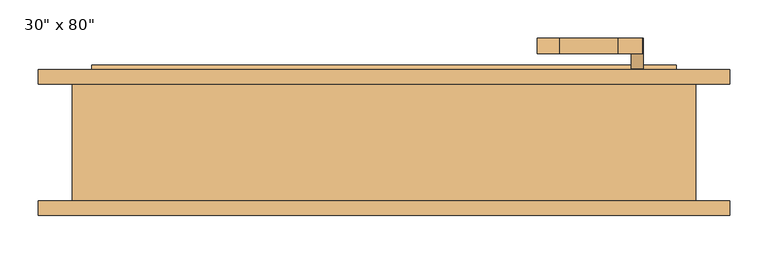
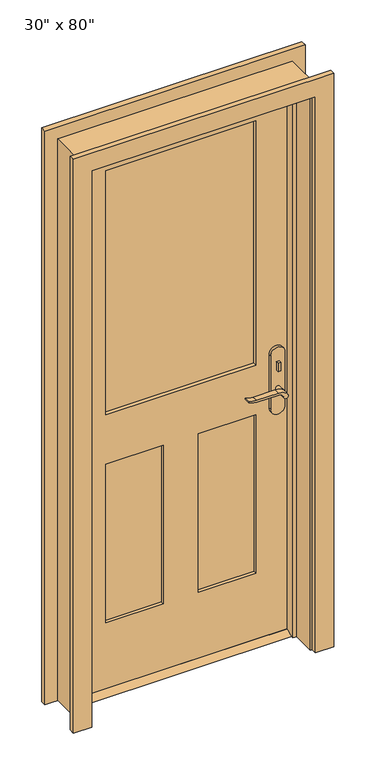
"""IFC4 building model written with IfcOpenShell, lengths in millimetres: door geometry."""

from ifc_helpers import new_model, si_unit, point, frame, frame_2d, origin, place, context, project, spatial, polyline, circle_curve, trimmed, segment, composite_curve, outline, extrude, faceted_brep, source, transform, mapped, element, save


def door_cdf9d6cc(model_context):
    return source(origin(), model_context, "Body", "SolidModel", [
        extrude(outline(polyline([(38.1, 12.7), (73.025, 12.7), (98.425, 0.0), (12.7, 0.0), (38.1, 12.7)])), frame((-381.0, 0.0, 0.0), z_axis=(1.0, 0.0, 0.0), x_axis=(0.0, 1.0, 0.0)), (0.0, 0.0, 1.0), 762.0),
        extrude(outline(polyline([(335.2, 18.1), (325.2, 18.1), (325.2, 28.1), (335.2, 28.1), (335.2, 18.1)])), frame((0.0, 0.0, 981.9), z_axis=(0.0, 0.0, 1.0), x_axis=(1.0, 0.0, 0.0)), (0.0, 0.0, 1.0), 30.0),
        extrude(outline(composite_curve([segment(trimmed(circle_curve(frame_2d((996.9, 330.2)), 8.0), [point((996.9, 322.2))], [point((996.9, 338.2))], False, "CARTESIAN"), True, "CONTINUOUS"), segment(trimmed(circle_curve(frame_2d((996.9, 330.2)), 8.0), [point((996.9, 338.2))], [point((996.9, 322.2))], False, "CARTESIAN"), True, "CONTINUOUS")], self_intersect=False)), frame((0.0, 83.025, 0.0), z_axis=(0.0, 1.0, 0.0), x_axis=(0.0, 0.0, 1.0)), (0.0, 0.0, 1.0), 10.0),
        extrude(outline(composite_curve([segment(trimmed(circle_curve(frame_2d((897.1555521, 306.5324871)), 37.2832219), [point((919.0523287, 336.7081363))], [point((934.4, 304.8325667))], False, "CARTESIAN"), True, "CONTINUOUS"), segment(polyline([(934.4, 304.8325667), (934.4, 228.5564091)]), True, "CONTINUOUS"), segment(trimmed(circle_curve(frame_2d((1017.6850638, 228.6227909)), 83.2850902), [point((934.4, 228.5564091))], [point((939.4, 200.2))], True, "CARTESIAN"), True, "CONTINUOUS"), segment(polyline([(939.4, 200.2), (936.6135558, 200.2)]), True, "CONTINUOUS"), segment(trimmed(circle_curve(frame_2d((986.6709207, 232.1396612)), 59.3791355), [point((936.6135558, 200.2))], [point((927.4, 228.5564091))], False, "CARTESIAN"), True, "CONTINUOUS"), segment(polyline([(927.4, 228.5564091), (927.4, 304.8138099)]), True, "CONTINUOUS"), segment(trimmed(circle_curve(frame_2d((909.2738613, 304.8138099)), 18.1261387), [point((927.4, 304.8138099))], [point((914.4, 322.2))], True, "CARTESIAN"), True, "CONTINUOUS"), segment(trimmed(circle_curve(frame_2d((914.4, 330.2)), 8.0), [point((914.4, 322.2))], [point((919.0523287, 336.7081363))], False, "CARTESIAN"), True, "CONTINUOUS")], self_intersect=False)), frame((0.0, -21.9, 0.0), z_axis=(0.0, 1.0, 0.0), x_axis=(0.0, 0.0, 1.0)), (0.0, 0.0, 1.0), 20.0),
        extrude(outline(composite_curve([segment(trimmed(circle_curve(frame_2d((914.4, 330.2)), 8.0), [point((914.3999903, 322.2))], [point((919.0523287, 336.7081363))], False, "CARTESIAN"), True, "CONTINUOUS"), segment(trimmed(circle_curve(frame_2d((897.1555521, 306.5324871)), 37.2832219), [point((919.0523287, 336.7081363))], [point((934.4, 304.8325667))], False, "CARTESIAN"), True, "CONTINUOUS"), segment(polyline([(934.4, 304.8325667), (934.4, 228.5564091)]), True, "CONTINUOUS"), segment(trimmed(circle_curve(frame_2d((1017.6850638, 228.6227909)), 83.2850902), [point((934.4, 228.5564091))], [point((939.4, 200.2))], True, "CARTESIAN"), True, "CONTINUOUS"), segment(polyline([(939.4, 200.2), (936.6135558, 200.2)]), True, "CONTINUOUS"), segment(trimmed(circle_curve(frame_2d((986.6709207, 232.1396612)), 59.3791355), [point((936.6135558, 200.2))], [point((927.4, 228.5564091))], False, "CARTESIAN"), True, "CONTINUOUS"), segment(polyline([(927.4, 228.5564091), (927.4, 304.8138122)]), True, "CONTINUOUS"), segment(trimmed(circle_curve(frame_2d((909.2738682, 304.8138122)), 18.1261318), [point((927.4, 304.8138122))], [point((914.3999903, 322.2))], True, "CARTESIAN"), True, "CONTINUOUS")], self_intersect=False)), frame((0.0, 113.025, 0.0), z_axis=(0.0, 1.0, 0.0), x_axis=(0.0, 0.0, 1.0)), (0.0, 0.0, 1.0), 20.0),
        extrude(outline(composite_curve([segment(trimmed(circle_curve(frame_2d((914.4, 330.2)), 8.0), [point((914.4, 322.2))], [point((914.4, 338.2))], False, "CARTESIAN"), True, "CONTINUOUS"), segment(trimmed(circle_curve(frame_2d((914.4, 330.2)), 8.0), [point((914.4, 338.2))], [point((914.4, 322.2))], False, "CARTESIAN"), True, "CONTINUOUS")], self_intersect=False)), frame((0.0, -1.9, 0.0), z_axis=(0.0, 1.0, 0.0), x_axis=(0.0, 0.0, 1.0)), (0.0, 0.0, 1.0), 30.0),
        extrude(outline(composite_curve([segment(trimmed(circle_curve(frame_2d((914.4, 330.2)), 8.0), [point((914.4, 322.2))], [point((914.4, 338.2))], False, "CARTESIAN"), True, "CONTINUOUS"), segment(trimmed(circle_curve(frame_2d((914.4, 330.2)), 8.0), [point((914.4, 338.2))], [point((914.4, 322.2))], False, "CARTESIAN"), True, "CONTINUOUS")], self_intersect=False)), frame((0.0, 83.025, 0.0), z_axis=(0.0, 1.0, 0.0), x_axis=(0.0, 0.0, 1.0)), (0.0, 0.0, 1.0), 30.0),
        extrude(outline(composite_curve([segment(polyline([(844.4, 355.2), (1039.4, 355.2)]), True, "CONTINUOUS"), segment(trimmed(circle_curve(frame_2d((1039.4, 330.2)), 25.0), [point((1039.4, 355.2))], [point((1039.4, 305.2))], False, "CARTESIAN"), True, "CONTINUOUS"), segment(polyline([(1039.4, 305.2), (844.4, 305.2)]), True, "CONTINUOUS"), segment(trimmed(circle_curve(frame_2d((844.4, 330.2)), 25.0), [point((844.4, 305.2))], [point((844.4, 355.2))], False, "CARTESIAN"), True, "CONTINUOUS")], self_intersect=False)), frame((0.0, 28.1, 0.0), z_axis=(0.0, 1.0, 0.0), x_axis=(0.0, 0.0, 1.0)), (0.0, 0.0, 1.0), 10.0),
        extrude(outline(composite_curve([segment(polyline([(844.4, 355.2), (1039.4, 355.2)]), True, "CONTINUOUS"), segment(trimmed(circle_curve(frame_2d((1039.4, 330.2)), 25.0), [point((1039.4, 355.2))], [point((1039.4, 305.2))], False, "CARTESIAN"), True, "CONTINUOUS"), segment(polyline([(1039.4, 305.2), (844.4, 305.2)]), True, "CONTINUOUS"), segment(trimmed(circle_curve(frame_2d((844.4, 330.2)), 25.0), [point((844.4, 305.2))], [point((844.4, 355.2))], False, "CARTESIAN"), True, "CONTINUOUS")], self_intersect=False)), frame((0.0, 73.025, 0.0), z_axis=(0.0, 1.0, 0.0), x_axis=(0.0, 0.0, 1.0)), (0.0, 0.0, 1.0), 10.0),
        extrude(outline(polyline([(2032.0, -381.0), (12.7, -381.0), (12.7, 381.0), (2032.0, 381.0), (2032.0, -381.0)]), holes=[polyline([(1016.0, -260.35), (1911.35, -260.35), (1911.35, 260.35), (1016.0, 260.35), (1016.0, -260.35)]), polyline([(835.025, -60.325), (254.0, -60.325), (254.0, -260.35), (835.025, -260.35), (835.025, -60.325)]), polyline([(835.025, 260.35), (254.0, 260.35), (254.0, 60.325), (835.025, 60.325), (835.025, 260.35)])]), frame((0.0, 38.1, 0.0), z_axis=(0.0, 1.0, 0.0), x_axis=(0.0, 0.0, 1.0)), (0.0, 0.0, 1.0), 34.925),
        faceted_brep([(406.4, 73.025, 0.0), (406.4, -79.375, 0.0), (381.0, -79.375, 0.0), (381.0, 3.175, 0.0), (368.3, 3.175, 0.0), (368.3, 38.1, 0.0), (381.0, 38.1, 0.0), (381.0, 73.025, 0.0), (406.4, 73.025, 2057.4), (406.4, -79.375, 2057.4), (-406.4, -79.375, 2057.4), (-406.4, -79.375, 0.0), (-381.0, -79.375, 0.0), (-381.0, -79.375, 2032.0), (381.0, -79.375, 2032.0), (381.0, 3.175, 2032.0), (-381.0, 3.175, 2032.0), (-381.0, 3.175, 0.0), (-368.3, 3.175, 0.0), (-368.3, 3.175, 2019.3), (368.3, 3.175, 2019.3), (368.3, 38.1, 2019.3), (-368.3, 38.1, 2019.3), (-368.3, 38.1, 0.0), (-381.0, 38.1, 0.0), (-381.0, 38.1, 2032.0), (381.0, 38.1, 2032.0), (381.0, 73.025, 2032.0), (-381.0, 73.025, 2032.0), (-381.0, 73.025, 0.0), (-406.4, 73.025, 0.0), (-406.4, 73.025, 2057.4)], [[[0, 1, 2, 3, 4, 5, 6, 7]], [[1, 0, 8, 9]], [[2, 1, 9, 10, 11, 12, 13, 14]], [[3, 2, 14, 15]], [[4, 3, 15, 16, 17, 18, 19, 20]], [[5, 4, 20, 21]], [[6, 5, 21, 22, 23, 24, 25, 26]], [[7, 6, 26, 27]], [[0, 7, 27, 28, 29, 30, 31, 8]], [[9, 8, 31, 10]], [[15, 14, 13, 16]], [[21, 20, 19, 22]], [[27, 26, 25, 28]], [[30, 29, 24, 23, 18, 17, 12, 11]], [[10, 31, 30, 11]], [[16, 13, 12, 17]], [[22, 19, 18, 23]], [[28, 25, 24, 29]]]),
        extrude(outline(polyline([(-60.325, 49.7416667), (-260.35, 49.7416667), (-260.35, 61.3833333), (-60.325, 61.3833333), (-60.325, 49.7416667)])), frame((0.0, 0.0, 254.0), z_axis=(0.0, 0.0, 1.0), x_axis=(1.0, 0.0, 0.0)), (0.0, 0.0, 1.0), 581.025),
        extrude(outline(polyline([(260.35, 49.7416667), (60.325, 49.7416667), (60.325, 61.3833333), (260.35, 61.3833333), (260.35, 49.7416667)])), frame((0.0, 0.0, 254.0), z_axis=(0.0, 0.0, 1.0), x_axis=(1.0, 0.0, 0.0)), (0.0, 0.0, 1.0), 581.025),
        extrude(outline(polyline([(260.35, 52.07), (-260.35, 52.07), (-260.35, 59.055), (260.35, 59.055), (260.35, 52.07)])), frame((0.0, 0.0, 1016.0), z_axis=(0.0, 0.0, 1.0), x_axis=(1.0, 0.0, 0.0)), (0.0, 0.0, 1.0), 895.35),
        extrude(outline(polyline([(0.0, -450.85), (0.0, -387.35), (2038.35, -387.35), (2038.35, 387.35), (0.0, 387.35), (0.0, 450.85), (2101.85, 450.85), (2101.85, -450.85), (0.0, -450.85)])), frame((0.0, -98.425, 0.0), z_axis=(0.0, 1.0, 0.0), x_axis=(0.0, 0.0, 1.0)), (0.0, 0.0, 1.0), 19.05),
        extrude(outline(polyline([(0.0, -450.85), (0.0, -387.35), (2038.35, -387.35), (2038.35, 387.35), (0.0, 387.35), (0.0, 450.85), (2101.85, 450.85), (2101.85, -450.85), (0.0, -450.85)])), frame((0.0, 73.025, 0.0), z_axis=(0.0, 1.0, 0.0), x_axis=(0.0, 0.0, 1.0)), (0.0, 0.0, 1.0), 19.05),
    ])


if __name__ == "__main__":
    model = new_model("IFC4")
    model_context = context("Model", 3, world=origin())
    ifc_project = project(units=[si_unit("LENGTHUNIT", "METRE", prefix="MILLI")], contexts=[model_context])
    site = spatial("IfcSite", under=ifc_project)
    building = spatial("IfcBuilding", under=site)
    placement = place(None, origin())
    door_shape = door_cdf9d6cc(model_context)
    element("IfcDoor", 1, ObjectType="30\" x 80\"", at=placement, inside=building, context=model_context, shape_type="MappedRepresentation", body=[
        mapped(door_shape, transform((0.0, 0.0, 0.0), x_axis=(1.0, 0.0, 0.0), y_axis=(0.0, 1.0, 0.0), z_axis=(0.0, 0.0, 1.0))),
    ])
    save(model, "model.ifc")

# Revit data of these elements
# Type "30\" x 80\""
#   Type Mark = "9"
#   Assembly Code = "B2030100"
#   Analytic Construction = "French door, wood frame with single glass"
#   Top Rail = 0' - 4 3/4"
#   Threshold Offset [instance default] = 0' - 0 1/2"
#   Thickness = 0' - 1 3/8"
#   Thermal Resistance (R) = 1.0696 (h·ft²·°F)/BTU
#   Swing Angle [instance default] = 90.00°
#   Stiles = 0' - 4 3/4"
#   Rough Width = 2' - 8"
#   Rough Height = 6' - 9"
#   Lock Rail = 0' - 7 1/8"
#   Height = 6' - 8"
#   Width = 2' - 6"
#   Heat Transfer Coefficient (U) = 0.9350 BTU/(h·ft²·°F)
#   Door Offset [instance default] = 0' - 0"
#   Bottom Rail = 0' - 9 1/2"
#   Threshold [instance default] = yes
#   Function = 1
#   Exterior Trim [instance default] = yes
#   Trim Material = Cherry
#   Threshold Material = Cherry
#   Panel Material = Cherry
#   Glazing = Glass
#   Frame Material = Cherry
#   Door Handle Material = Aluminum
#   Visual Light Transmittance = 0
#   Solar Heat Gain Coefficient = 0
#   Wall Closure = (empty or 0)
#   Construction Type = (empty or 0)
# Element 1 (IfcDoor, "30\" x 80\"")
#   Materials on its faces: "Cherry", "Aluminum", "Glass"
# Materials
#   "Cherry": class "Wood", colour RGB 226 177 128, transparency 0, Description = "Prunus Serotina", Cost = 0
#   "Glass": class "Glass", colour RGB 0 128 192, transparency 0.75, Description = "Soda Lime Glass", Cost = 0
#   "Aluminum": class "Metal", colour RGB 247 247 247, transparency 0, Description = "Aluminum 6061", Cost = 0
